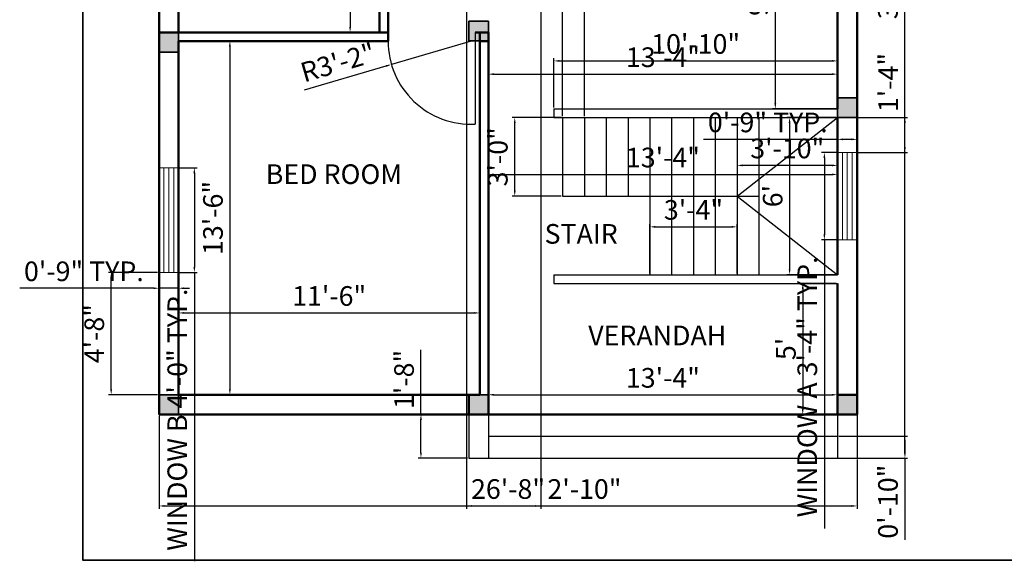
# Model space of a CAD drawing. Units: inches. Extents: x 2289 to 3796, y 1741 to 2286.
# Tile 1 of 4: x 2289 to 2741, y 1741 to 1989. Entities that reach past the tile are written whole.
import ezdxf

# ---------------------------------------------------------------- set-up
doc = ezdxf.new("R2010")
doc.units = ezdxf.units.IN
for name, color, linetype, lineweight in [('A-ANNO-DIMS', 2, 'Continuous', 18), ('A-ANNO-TTLB', 7, 'Continuous', 35), ('A-AREA-IDEN', 7, 'Continuous', 25), ('A-DOOR', 3, 'Continuous', 25), ('A-FLOR-STRS', 7, 'Continuous', 25), ('A-GLAZ', 4, 'Continuous', 18), ('A-WALL', 7, 'Continuous', 50), ('S-COLS', 1, 'Continuous', 35)]:
    doc.layers.add(name, color=color, linetype=linetype, lineweight=lineweight)
doc.styles.get("Standard").update_dxf_attribs({"font": 'arial.ttf'})
doc.dimstyles.new('ISO-25', dxfattribs={"dimtxt": 9, "dimasz": 2.5, "dimexe": 1.25, "dimexo": 0.625, "dimgap": 2, "dimtad": 1, "dimdec": 1, "dimlunit": 4, "dimtxsty": 'Standard', "dimcen": 2.5, "dimadec": 0, "dimazin": 0, "dimtfac": 1, "dimtdec": 1, "dimtmove": 0, "dimatfit": 3, "dimfxl": 1, "dimarcsym": 0})

# ---------------------------------------------------------------- blocks, each defined once
blk = doc.blocks.new('*D7')
at = {"layer": 'A-ANNO-DIMS', "color": 0, "lineweight": -2, "transparency": 16777216}
for p, q in [((2362.08, 1818.01), (2362.08, 1856.13)), ((2500.08, 1818.01), (2500.08, 1856.13)), ((2364.58, 1854.88), (2497.58, 1854.88))]:
    blk.add_line(p, q, dxfattribs=at)
at = {"layer": 'A-ANNO-DIMS', "color": 0, "transparency": 16777216}
for points in [[(2364.58, 1855.3), (2364.58, 1854.46), (2362.08, 1854.88)], [(2497.58, 1855.3), (2497.58, 1854.46), (2500.08, 1854.88)]]:
    blk.add_solid(points, dxfattribs=at)
at = {"layer": 'Defpoints', "color": 0, "transparency": 16777216}
for p in [(2500.08, 1854.88), (2362.08, 1817.39), (2500.08, 1817.39)]:
    blk.add_point(p, dxfattribs=at)
at = {"layer": 'A-ANNO-DIMS', "color": 0, "transparency": 16777216, "insert": (2431.08, 1861.48), "char_height": 9, "attachment_point": 5}
blk.add_mtext('11\'-6"', dxfattribs=at)
blk = doc.blocks.new('*D8')
at = {"layer": 'A-ANNO-DIMS', "color": 0, "lineweight": -2, "transparency": 16777216}
for p, q in [((2362.7, 1979.39), (2386.82, 1979.39)), ((2385.57, 1976.89), (2385.57, 1819.89)), ((2362.7, 1817.39), (2386.82, 1817.39))]:
    blk.add_line(p, q, dxfattribs=at)
at = {"layer": 'A-ANNO-DIMS', "color": 0, "transparency": 16777216}
for points in [[(2385.16, 1976.89), (2385.99, 1976.89), (2385.57, 1979.39)], [(2385.16, 1819.89), (2385.99, 1819.89), (2385.57, 1817.39)]]:
    blk.add_solid(points, dxfattribs=at)
at = {"layer": 'Defpoints', "color": 0, "transparency": 16777216}
for p in [(2362.08, 1979.39), (2362.08, 1817.39), (2385.57, 1817.39)]:
    blk.add_point(p, dxfattribs=at)
at = {"layer": 'A-ANNO-DIMS', "color": 0, "transparency": 16777216, "insert": (2378.98, 1898.39), "char_height": 9, "attachment_point": 5, "rotation": 90}
blk.add_mtext('13\'-6"', dxfattribs=at)
blk = doc.blocks.new('*D9')
at = {"layer": 'A-ANNO-DIMS', "color": 0, "lineweight": -2, "transparency": 16777216}
for p, q in [((2504.08, 1867.76), (2504.08, 1816.14)), ((2664.08, 1867.76), (2664.08, 1816.14)), ((2506.58, 1817.39), (2661.58, 1817.39))]:
    blk.add_line(p, q, dxfattribs=at)
at = {"layer": 'A-ANNO-DIMS', "color": 0, "transparency": 16777216}
for points in [[(2506.58, 1817.8), (2506.58, 1816.97), (2504.08, 1817.39)], [(2661.58, 1817.8), (2661.58, 1816.97), (2664.08, 1817.39)]]:
    blk.add_solid(points, dxfattribs=at)
at = {"layer": 'Defpoints', "color": 0, "transparency": 16777216}
for p in [(2504.08, 1868.39), (2664.08, 1868.39), (2664.08, 1817.39)]:
    blk.add_point(p, dxfattribs=at)
at = {"layer": 'A-ANNO-DIMS', "color": 0, "transparency": 16777216, "insert": (2584.08, 1823.98), "char_height": 9, "attachment_point": 5}
blk.add_mtext('13\'-4"', dxfattribs=at)
blk = doc.blocks.new('*D10')
at = {"layer": 'A-ANNO-DIMS', "color": 0, "lineweight": -2, "transparency": 16777216}
for p, q in [((2663.45, 1868.39), (2646.93, 1868.39)), ((2648.18, 1865.89), (2648.18, 1810.89)), ((2663.45, 1808.39), (2646.93, 1808.39))]:
    blk.add_line(p, q, dxfattribs=at)
at = {"layer": 'A-ANNO-DIMS', "color": 0, "transparency": 16777216}
for points in [[(2647.76, 1865.89), (2648.6, 1865.89), (2648.18, 1868.39)], [(2647.76, 1810.89), (2648.6, 1810.89), (2648.18, 1808.39)]]:
    blk.add_solid(points, dxfattribs=at)
at = {"layer": 'Defpoints', "color": 0, "transparency": 16777216}
for p in [(2664.08, 1868.39), (2648.18, 1808.39), (2664.08, 1808.39)]:
    blk.add_point(p, dxfattribs=at)
at = {"layer": 'A-ANNO-DIMS', "color": 0, "transparency": 16777216, "insert": (2641.6, 1838.39), "char_height": 9, "attachment_point": 5, "rotation": 90}
blk.add_mtext("5'", dxfattribs=at)
blk = doc.blocks.new('*D11')
at = {"layer": 'A-ANNO-DIMS', "color": 0, "lineweight": -2, "transparency": 16777216}
for p, q in [((2504.08, 1873.01), (2504.08, 1919.55)), ((2506.58, 1918.3), (2661.58, 1918.3)), ((2664.08, 1873.01), (2664.08, 1919.55))]:
    blk.add_line(p, q, dxfattribs=at)
at = {"layer": 'A-ANNO-DIMS', "color": 0, "transparency": 16777216}
for points in [[(2506.58, 1918.72), (2506.58, 1917.89), (2504.08, 1918.3)], [(2661.58, 1918.72), (2661.58, 1917.89), (2664.08, 1918.3)]]:
    blk.add_solid(points, dxfattribs=at)
at = {"layer": 'Defpoints', "color": 0, "transparency": 16777216}
for p in [(2664.08, 1918.3), (2504.08, 1872.39), (2664.08, 1872.39)]:
    blk.add_point(p, dxfattribs=at)
at = {"layer": 'A-ANNO-DIMS', "color": 0, "transparency": 16777216, "insert": (2584.08, 1924.9), "char_height": 9, "attachment_point": 5}
blk.add_mtext('13\'-4"', dxfattribs=at)
blk = doc.blocks.new('*D12')
at = {"layer": 'A-ANNO-DIMS', "color": 0, "lineweight": -2, "transparency": 16777216}
for p, q in [((2663.45, 1944.39), (2640.9, 1944.39)), ((2642.15, 1941.89), (2642.15, 1874.89)), ((2663.45, 1872.39), (2640.9, 1872.39))]:
    blk.add_line(p, q, dxfattribs=at)
at = {"layer": 'A-ANNO-DIMS', "color": 0, "transparency": 16777216}
for points in [[(2641.73, 1941.89), (2642.56, 1941.89), (2642.15, 1944.39)], [(2641.73, 1874.89), (2642.56, 1874.89), (2642.15, 1872.39)]]:
    blk.add_solid(points, dxfattribs=at)
at = {"layer": 'Defpoints', "color": 0, "transparency": 16777216}
for p in [(2664.08, 1944.39), (2642.15, 1872.39), (2664.08, 1872.39)]:
    blk.add_point(p, dxfattribs=at)
at = {"layer": 'A-ANNO-DIMS', "color": 0, "transparency": 16777216, "insert": (2635.55, 1908.39), "char_height": 9, "attachment_point": 5, "rotation": 90}
blk.add_mtext("6'", dxfattribs=at)
blk = doc.blocks.new('*D13')
at = {"layer": 'A-ANNO-DIMS', "color": 0, "lineweight": -2, "transparency": 16777216}
for p, q in [((2664.08, 2007.26), (2664.08, 1963)), ((2504.08, 1978.76), (2504.08, 1963)), ((2506.58, 1964.25), (2661.58, 1964.25))]:
    blk.add_line(p, q, dxfattribs=at)
at = {"layer": 'A-ANNO-DIMS', "color": 0, "transparency": 16777216}
for points in [[(2506.58, 1964.67), (2506.58, 1963.83), (2504.08, 1964.25)], [(2661.58, 1964.67), (2661.58, 1963.83), (2664.08, 1964.25)]]:
    blk.add_solid(points, dxfattribs=at)
at = {"layer": 'Defpoints', "color": 0, "transparency": 16777216}
for p in [(2664.08, 2007.89), (2504.08, 1979.39), (2664.08, 1964.25)]:
    blk.add_point(p, dxfattribs=at)
at = {"layer": 'A-ANNO-DIMS', "color": 0, "transparency": 16777216, "insert": (2584.08, 1970.85), "char_height": 9, "attachment_point": 5}
blk.add_mtext('13\'-4"', dxfattribs=at)
blk = doc.blocks.new('*D14')
at = {"layer": 'A-ANNO-DIMS', "color": 0, "lineweight": -2, "transparency": 16777216}
for p, q in [((2362.7, 2067.39), (2441.94, 2067.39)), ((2440.69, 2064.89), (2440.69, 1985.89)), ((2362.7, 1983.39), (2441.94, 1983.39))]:
    blk.add_line(p, q, dxfattribs=at)
at = {"layer": 'A-ANNO-DIMS', "color": 0, "transparency": 16777216}
for points in [[(2440.27, 2064.89), (2441.1, 2064.89), (2440.69, 2067.39)], [(2440.27, 1985.89), (2441.1, 1985.89), (2440.69, 1983.39)]]:
    blk.add_solid(points, dxfattribs=at)
at = {"layer": 'Defpoints', "color": 0, "transparency": 16777216}
for p in [(2362.08, 2067.39), (2362.08, 1983.39), (2440.69, 1983.39)]:
    blk.add_point(p, dxfattribs=at)
at = {"layer": 'A-ANNO-DIMS', "color": 0, "transparency": 16777216, "insert": (2434.19, 2025.39), "char_height": 9, "attachment_point": 5, "rotation": 90}
blk.add_mtext("7'", dxfattribs=at)
blk = doc.blocks.new('*D15')
at = {"layer": 'A-ANNO-DIMS', "color": 0, "lineweight": -2, "transparency": 16777216}
for p, q in [((2663.45, 2067.39), (2634.35, 2067.39)), ((2635.6, 2064.89), (2635.6, 1950.89)), ((2663.45, 1948.39), (2634.35, 1948.39))]:
    blk.add_line(p, q, dxfattribs=at)
at = {"layer": 'A-ANNO-DIMS', "color": 0, "transparency": 16777216}
for points in [[(2635.18, 2064.89), (2636.02, 2064.89), (2635.6, 2067.39)], [(2635.18, 1950.89), (2636.02, 1950.89), (2635.6, 1948.39)]]:
    blk.add_solid(points, dxfattribs=at)
at = {"layer": 'Defpoints', "color": 0, "transparency": 16777216}
for p in [(2664.08, 2067.39), (2635.6, 1948.39), (2664.08, 1948.39)]:
    blk.add_point(p, dxfattribs=at)
at = {"layer": 'A-ANNO-DIMS', "color": 0, "transparency": 16777216, "insert": (2629, 2007.89), "char_height": 9, "attachment_point": 5, "rotation": 90}
blk.add_mtext('9\'-11"', dxfattribs=at)
blk = doc.blocks.new('WIN-40IN')
for p, q in [((0, 40), (9, 40)), ((2.25, 40), (2.25, 0)), ((4.5, 40), (4.5, 0)), ((6.75, 40), (6.75, 0)), ((0, 0), (9, 0))]:
    blk.add_line(p, q)
blk = doc.blocks.new('WIN-48IN')
for p, q in [((0, 48), (9, 48)), ((2.25, 48), (2.25, 0)), ((4.5, 48), (4.5, 0)), ((6.75, 48), (6.75, 0)), ((0, 0), (9, 0))]:
    blk.add_line(p, q)
blk = doc.blocks.new('COL-9X9')
h = blk.add_hatch(color=256)
h.dxf.hatch_style = 1
h.paths.add_polyline_path([(0, 9), (0, 0), (9, 0), (9, 9)])
blk.add_lwpolyline([(0, 9), (9, 9), (9, 0), (0, 0)], close=True)
blk = doc.blocks.new('COL-9X9-STAIR')
h = blk.add_hatch(color=256)
h.dxf.hatch_style = 1
h.paths.add_polyline_path([(9, 0), (9, 9), (0, 9), (0, 0)])
blk.add_lwpolyline([(0.01, 9.14), (9.01, 9.14), (9.01, 0.14), (0.01, 0.14)], close=True)
blk = doc.blocks.new('*D31')
at = {"layer": 'A-ANNO-DIMS', "color": 0, "lineweight": -2, "transparency": 16777216}
for p, q in [((2663.45, 1928.39), (2656.83, 1928.39)), ((2658.08, 1925.89), (2658.08, 1890.89)), ((2663.45, 1888.39), (2656.83, 1888.39)), ((2658.08, 1888.39), (2658.08, 1756.12))]:
    blk.add_line(p, q, dxfattribs=at)
at = {"layer": 'A-ANNO-DIMS', "color": 0, "transparency": 16777216}
for points in [[(2657.66, 1925.89), (2658.49, 1925.89), (2658.08, 1928.39)], [(2657.66, 1890.89), (2658.49, 1890.89), (2658.08, 1888.39)]]:
    blk.add_solid(points, dxfattribs=at)
at = {"layer": 'Defpoints', "color": 0, "transparency": 16777216}
for p in [(2664.08, 1928.39), (2658.08, 1888.39), (2664.08, 1888.39)]:
    blk.add_point(p, dxfattribs=at)
at = {"layer": 'A-ANNO-DIMS', "color": 0, "transparency": 16777216, "insert": (2651.42, 1821), "char_height": 9, "attachment_point": 5, "rotation": 90}
blk.add_mtext('WINDOW A 3\'-4" TYP.', dxfattribs=at)
blk = doc.blocks.new('*D32')
at = {"layer": 'A-ANNO-DIMS', "color": 0, "lineweight": -2, "transparency": 16777216}
for p, q in [((2664.08, 1934.39), (2602.72, 1934.39)), ((2664.08, 1929.01), (2664.08, 1935.64)), ((2670.58, 1934.39), (2666.58, 1934.39)), ((2673.08, 1929.01), (2673.08, 1935.64))]:
    blk.add_line(p, q, dxfattribs=at)
at = {"layer": 'A-ANNO-DIMS', "color": 0, "transparency": 16777216}
for points in [[(2666.58, 1934.8), (2666.58, 1933.97), (2664.08, 1934.39)], [(2670.58, 1934.8), (2670.58, 1933.97), (2673.08, 1934.39)]]:
    blk.add_solid(points, dxfattribs=at)
at = {"layer": 'Defpoints', "color": 0, "transparency": 16777216}
for p in [(2664.08, 1934.39), (2664.08, 1928.39), (2673.08, 1928.39)]:
    blk.add_point(p, dxfattribs=at)
at = {"layer": 'A-ANNO-DIMS', "color": 0, "transparency": 16777216, "insert": (2632.15, 1940.98), "char_height": 9, "attachment_point": 5}
blk.add_mtext('0\'-9" TYP.', dxfattribs=at)
blk = doc.blocks.new('*D33')
at = {"layer": 'A-ANNO-DIMS', "color": 0, "lineweight": -2, "transparency": 16777216}
for p, q in [((2362.7, 1921.39), (2370.53, 1921.39)), ((2369.28, 1918.89), (2369.28, 1875.89)), ((2362.7, 1873.39), (2370.53, 1873.39)), ((2369.28, 1873.39), (2369.28, 1741.12))]:
    blk.add_line(p, q, dxfattribs=at)
at = {"layer": 'A-ANNO-DIMS', "color": 0, "transparency": 16777216}
for points in [[(2368.86, 1918.89), (2369.69, 1918.89), (2369.28, 1921.39)], [(2368.86, 1875.89), (2369.69, 1875.89), (2369.28, 1873.39)]]:
    blk.add_solid(points, dxfattribs=at)
at = {"layer": 'Defpoints', "color": 0, "transparency": 16777216}
for p in [(2362.08, 1921.39), (2362.08, 1873.39), (2369.28, 1873.39)]:
    blk.add_point(p, dxfattribs=at)
at = {"layer": 'A-ANNO-DIMS', "color": 0, "transparency": 16777216, "insert": (2362.62, 1806), "char_height": 9, "attachment_point": 5, "rotation": 90}
blk.add_mtext('WINDOW B 4\'-0" TYP.', dxfattribs=at)
blk = doc.blocks.new('*D34')
at = {"layer": 'A-ANNO-DIMS', "color": 0, "lineweight": -2, "transparency": 16777216}
for p, q in [((2353.08, 1872.76), (2353.08, 1864.94)), ((2362.08, 1872.76), (2362.08, 1864.94)), ((2350.58, 1866.19), (2289.22, 1866.19)), ((2362.08, 1866.19), (2353.08, 1866.19)), ((2364.58, 1866.19), (2367.08, 1866.19))]:
    blk.add_line(p, q, dxfattribs=at)
at = {"layer": 'A-ANNO-DIMS', "color": 0, "transparency": 16777216}
for points in [[(2350.58, 1866.6), (2350.58, 1865.77), (2353.08, 1866.19)], [(2364.58, 1866.6), (2364.58, 1865.77), (2362.08, 1866.19)]]:
    blk.add_solid(points, dxfattribs=at)
at = {"layer": 'Defpoints', "color": 0, "transparency": 16777216}
for p in [(2353.08, 1873.39), (2362.08, 1873.39), (2353.08, 1866.19)]:
    blk.add_point(p, dxfattribs=at)
at = {"layer": 'A-ANNO-DIMS', "color": 0, "transparency": 16777216, "insert": (2318.65, 1872.78), "char_height": 9, "attachment_point": 5}
blk.add_mtext('0\'-9" TYP.', dxfattribs=at)
blk = doc.blocks.new('*D35')
at = {"layer": 'A-ANNO-DIMS', "color": 0, "lineweight": -2, "transparency": 16777216}
for p, q in [((2353.08, 1807.76), (2353.08, 1765.21)), ((2673.08, 1787.76), (2673.08, 1765.21)), ((2355.58, 1766.46), (2670.58, 1766.46))]:
    blk.add_line(p, q, dxfattribs=at)
at = {"layer": 'A-ANNO-DIMS', "color": 0, "transparency": 16777216}
for points in [[(2355.58, 1766.88), (2355.58, 1766.04), (2353.08, 1766.46)], [(2670.58, 1766.88), (2670.58, 1766.04), (2673.08, 1766.46)]]:
    blk.add_solid(points, dxfattribs=at)
at = {"layer": 'Defpoints', "color": 0, "transparency": 16777216}
for p in [(2353.08, 1808.39), (2673.08, 1788.39), (2673.08, 1766.46)]:
    blk.add_point(p, dxfattribs=at)
at = {"layer": 'A-ANNO-DIMS', "color": 0, "transparency": 16777216, "insert": (2513.08, 1773.06), "char_height": 9, "attachment_point": 5}
blk.add_mtext('26\'-8"', dxfattribs=at)
blk = doc.blocks.new('*D36')
at = {"layer": 'A-ANNO-DIMS', "color": 0, "lineweight": -2, "transparency": 16777216}
for p, q in [((2673.7, 2224.39), (2696.25, 2224.39)), ((2695, 1790.89), (2695, 2221.89)), ((2673.7, 1788.39), (2696.25, 1788.39))]:
    blk.add_line(p, q, dxfattribs=at)
at = {"layer": 'A-ANNO-DIMS', "color": 0, "transparency": 16777216}
for points in [[(2694.59, 2221.89), (2695.42, 2221.89), (2695, 2224.39)], [(2694.59, 1790.89), (2695.42, 1790.89), (2695, 1788.39)]]:
    blk.add_solid(points, dxfattribs=at)
at = {"layer": 'Defpoints', "color": 0, "transparency": 16777216}
for p in [(2673.08, 2224.39), (2695, 2224.39), (2673.08, 1788.39)]:
    blk.add_point(p, dxfattribs=at)
at = {"layer": 'A-ANNO-DIMS', "color": 0, "transparency": 16777216, "insert": (2688.4, 2006.39), "char_height": 9, "attachment_point": 5, "rotation": 90}
blk.add_mtext('36\'-4"', dxfattribs=at)
blk = doc.blocks.new('*D37')
at = {"layer": 'A-ANNO-DIMS', "color": 0, "lineweight": -2, "transparency": 16777216}
for p, q in [((2473.15, 1808.39), (2473.15, 1837.96)), ((2494.45, 1808.39), (2471.9, 1808.39)), ((2473.15, 1790.89), (2473.15, 1805.89)), ((2494.45, 1788.39), (2471.9, 1788.39))]:
    blk.add_line(p, q, dxfattribs=at)
at = {"layer": 'A-ANNO-DIMS', "color": 0, "transparency": 16777216}
for points in [[(2472.74, 1805.89), (2473.57, 1805.89), (2473.15, 1808.39)], [(2472.74, 1790.89), (2473.57, 1790.89), (2473.15, 1788.39)]]:
    blk.add_solid(points, dxfattribs=at)
at = {"layer": 'Defpoints', "color": 0, "transparency": 16777216}
for p in [(2473.15, 1808.39), (2495.08, 1808.39), (2495.08, 1788.39)]:
    blk.add_point(p, dxfattribs=at)
at = {"layer": 'A-ANNO-DIMS', "color": 0, "transparency": 16777216, "insert": (2466.56, 1824.42), "char_height": 9, "attachment_point": 5, "rotation": 90}
blk.add_mtext('1\'-8"', dxfattribs=at)
blk = doc.blocks.new('*D40')
at = {"layer": 'A-ANNO-DIMS', "color": 0, "lineweight": -2, "transparency": 16777216}
for p, q in [((2352.45, 1873.39), (2329.9, 1873.39)), ((2331.15, 1819.89), (2331.15, 1870.89)), ((2352.45, 1817.39), (2329.9, 1817.39))]:
    blk.add_line(p, q, dxfattribs=at)
at = {"layer": 'A-ANNO-DIMS', "color": 0, "transparency": 16777216}
for points in [[(2330.74, 1870.89), (2331.57, 1870.89), (2331.15, 1873.39)], [(2330.74, 1819.89), (2331.57, 1819.89), (2331.15, 1817.39)]]:
    blk.add_solid(points, dxfattribs=at)
at = {"layer": 'Defpoints', "color": 0, "transparency": 16777216}
for p in [(2331.15, 1873.39), (2353.08, 1873.39), (2353.08, 1817.39)]:
    blk.add_point(p, dxfattribs=at)
at = {"layer": 'A-ANNO-DIMS', "color": 0, "transparency": 16777216, "insert": (2324.56, 1845.39), "char_height": 9, "attachment_point": 5, "rotation": 90}
blk.add_mtext('4\'-8"', dxfattribs=at)
blk = doc.blocks.new('*D43')
at = {"layer": 'A-ANNO-DIMS', "color": 0, "lineweight": -2, "transparency": 16777216}
for p, q in [((2695, 1944.39), (2695, 1973.96)), ((2673.7, 1944.39), (2696.25, 1944.39)), ((2695, 1930.89), (2695, 1941.89)), ((2673.7, 1928.39), (2696.25, 1928.39))]:
    blk.add_line(p, q, dxfattribs=at)
at = {"layer": 'A-ANNO-DIMS', "color": 0, "transparency": 16777216}
for points in [[(2694.59, 1941.89), (2695.42, 1941.89), (2695, 1944.39)], [(2694.59, 1930.89), (2695.42, 1930.89), (2695, 1928.39)]]:
    blk.add_solid(points, dxfattribs=at)
at = {"layer": 'Defpoints', "color": 0, "transparency": 16777216}
for p in [(2673.08, 1944.39), (2695, 1944.39), (2673.08, 1928.39)]:
    blk.add_point(p, dxfattribs=at)
at = {"layer": 'A-ANNO-DIMS', "color": 0, "transparency": 16777216, "insert": (2688.48, 1960.42), "char_height": 9, "attachment_point": 5, "rotation": 90}
blk.add_mtext('1\'-4"', dxfattribs=at)
blk = doc.blocks.new('*D46')
at = {"layer": 'A-ANNO-DIMS', "color": 0, "lineweight": -2, "transparency": 16777216}
for p, q in [((2494.08, 2126.76), (2494.08, 1765.21)), ((2528.08, 2126.76), (2528.08, 1765.21)), ((2496.58, 1766.46), (2525.58, 1766.46)), ((2528.08, 1766.46), (2565.65, 1766.46))]:
    blk.add_line(p, q, dxfattribs=at)
at = {"layer": 'A-ANNO-DIMS', "color": 0, "transparency": 16777216}
for points in [[(2496.58, 1766.88), (2496.58, 1766.04), (2494.08, 1766.46)], [(2525.58, 1766.88), (2525.58, 1766.04), (2528.08, 1766.46)]]:
    blk.add_solid(points, dxfattribs=at)
at = {"layer": 'Defpoints', "color": 0, "transparency": 16777216}
for p in [(2494.08, 2127.39), (2528.08, 2127.39), (2528.08, 1766.46)]:
    blk.add_point(p, dxfattribs=at)
at = {"layer": 'A-ANNO-DIMS', "color": 0, "transparency": 16777216, "insert": (2548.11, 1773.06), "char_height": 9, "attachment_point": 5}
blk.add_mtext('2\'-10"', dxfattribs=at)
blk = doc.blocks.new('*D48')
at = {"layer": 'A-ANNO-DIMS', "color": 0, "lineweight": -2, "transparency": 16777216}
for p, q in [((2538.08, 1945.01), (2538.08, 2247.56)), ((2540.58, 2246.31), (2545.58, 2246.31)), ((2548.08, 1945.01), (2548.08, 2247.56)), ((2548.08, 2246.31), (2585.49, 2246.31))]:
    blk.add_line(p, q, dxfattribs=at)
at = {"layer": 'A-ANNO-DIMS', "color": 0, "transparency": 16777216}
for points in [[(2540.58, 2246.73), (2540.58, 2245.89), (2538.08, 2246.31)], [(2545.58, 2246.73), (2545.58, 2245.89), (2548.08, 2246.31)]]:
    blk.add_solid(points, dxfattribs=at)
at = {"layer": 'Defpoints', "color": 0, "transparency": 16777216}
for p in [(2548.08, 2246.31), (2538.08, 1944.39), (2548.08, 1944.39)]:
    blk.add_point(p, dxfattribs=at)
at = {"layer": 'A-ANNO-DIMS', "color": 0, "transparency": 16777216, "insert": (2568.04, 2252.91), "char_height": 9, "attachment_point": 5}
blk.add_mtext('0\'-10"', dxfattribs=at)
blk = doc.blocks.new('*D49')
at = {"layer": 'A-ANNO-DIMS', "color": 0, "lineweight": -2, "transparency": 16777216}
for p, q in [((2537.45, 1944.39), (2514.9, 1944.39)), ((2516.15, 1910.89), (2516.15, 1941.89)), ((2537.45, 1908.39), (2514.9, 1908.39))]:
    blk.add_line(p, q, dxfattribs=at)
at = {"layer": 'A-ANNO-DIMS', "color": 0, "transparency": 16777216}
for points in [[(2515.74, 1941.89), (2516.57, 1941.89), (2516.15, 1944.39)], [(2515.74, 1910.89), (2516.57, 1910.89), (2516.15, 1908.39)]]:
    blk.add_solid(points, dxfattribs=at)
at = {"layer": 'Defpoints', "color": 0, "transparency": 16777216}
for p in [(2516.15, 1944.39), (2538.08, 1944.39), (2538.08, 1908.39)]:
    blk.add_point(p, dxfattribs=at)
at = {"layer": 'A-ANNO-DIMS', "color": 0, "transparency": 16777216, "insert": (2509.55, 1926.39), "char_height": 9, "attachment_point": 5, "rotation": 90}
blk.add_mtext('3\'-0"', dxfattribs=at)
blk = doc.blocks.new('*D50')
at = {"layer": 'A-ANNO-DIMS', "color": 0, "lineweight": -2, "transparency": 16777216}
for p, q in [((2618.08, 1943.76), (2618.08, 1921.21)), ((2664.08, 1943.76), (2664.08, 1921.21)), ((2661.58, 1922.46), (2620.58, 1922.46))]:
    blk.add_line(p, q, dxfattribs=at)
at = {"layer": 'A-ANNO-DIMS', "color": 0, "transparency": 16777216}
for points in [[(2620.58, 1922.88), (2620.58, 1922.04), (2618.08, 1922.46)], [(2661.58, 1922.88), (2661.58, 1922.04), (2664.08, 1922.46)]]:
    blk.add_solid(points, dxfattribs=at)
at = {"layer": 'Defpoints', "color": 0, "transparency": 16777216}
for p in [(2618.08, 1944.39), (2664.08, 1944.39), (2618.08, 1922.46)]:
    blk.add_point(p, dxfattribs=at)
at = {"layer": 'A-ANNO-DIMS', "color": 0, "transparency": 16777216, "insert": (2641.08, 1929.06), "char_height": 9, "attachment_point": 5}
blk.add_mtext('3\'-10"', dxfattribs=at)
blk = doc.blocks.new('*D51')
at = {"layer": 'A-ANNO-DIMS', "color": 0, "lineweight": -2, "transparency": 16777216}
for p, q in [((2578.08, 1873.01), (2578.08, 1895.56)), ((2580.58, 1894.31), (2615.58, 1894.31)), ((2618.08, 1873.01), (2618.08, 1895.56))]:
    blk.add_line(p, q, dxfattribs=at)
at = {"layer": 'A-ANNO-DIMS', "color": 0, "transparency": 16777216}
for points in [[(2580.58, 1894.73), (2580.58, 1893.89), (2578.08, 1894.31)], [(2615.58, 1894.73), (2615.58, 1893.89), (2618.08, 1894.31)]]:
    blk.add_solid(points, dxfattribs=at)
at = {"layer": 'Defpoints', "color": 0, "transparency": 16777216}
for p in [(2618.08, 1894.31), (2578.08, 1872.39), (2618.08, 1872.39)]:
    blk.add_point(p, dxfattribs=at)
at = {"layer": 'A-ANNO-DIMS', "color": 0, "transparency": 16777216, "insert": (2598.08, 1900.91), "char_height": 9, "attachment_point": 5}
blk.add_mtext('3\'-4"', dxfattribs=at)
blk = doc.blocks.new('*D52')
at = {"layer": 'A-ANNO-DIMS', "color": 0, "lineweight": -2, "transparency": 16777216}
for p, q in [((2534.08, 1949.01), (2534.08, 1971.56)), ((2536.58, 1970.31), (2661.58, 1970.31)), ((2664.08, 1949.01), (2664.08, 1971.56))]:
    blk.add_line(p, q, dxfattribs=at)
at = {"layer": 'A-ANNO-DIMS', "color": 0, "transparency": 16777216}
for points in [[(2536.58, 1970.73), (2536.58, 1969.89), (2534.08, 1970.31)], [(2661.58, 1970.73), (2661.58, 1969.89), (2664.08, 1970.31)]]:
    blk.add_solid(points, dxfattribs=at)
at = {"layer": 'Defpoints', "color": 0, "transparency": 16777216}
for p in [(2664.08, 1970.31), (2534.08, 1948.39), (2664.08, 1948.39)]:
    blk.add_point(p, dxfattribs=at)
at = {"layer": 'A-ANNO-DIMS', "color": 0, "transparency": 16777216, "insert": (2599.08, 1976.91), "char_height": 9, "attachment_point": 5}
blk.add_mtext('10\'-10"', dxfattribs=at)
blk = doc.blocks.new('*D53')
at = {"layer": 'A-ANNO-DIMS', "color": 0, "lineweight": -2, "transparency": 16777216}
for p, q in [((2664.7, 1798.39), (2696.25, 1798.39)), ((2695, 1795.89), (2695, 1790.89)), ((2664.7, 1788.39), (2696.25, 1788.39)), ((2695, 1788.39), (2695, 1750.97))]:
    blk.add_line(p, q, dxfattribs=at)
at = {"layer": 'A-ANNO-DIMS', "color": 0, "transparency": 16777216}
for points in [[(2694.59, 1795.89), (2695.42, 1795.89), (2695, 1798.39)], [(2694.59, 1790.89), (2695.42, 1790.89), (2695, 1788.39)]]:
    blk.add_solid(points, dxfattribs=at)
at = {"layer": 'Defpoints', "color": 0, "transparency": 16777216}
for p in [(2664.08, 1798.39), (2664.08, 1788.39), (2695, 1788.39)]:
    blk.add_point(p, dxfattribs=at)
at = {"layer": 'A-ANNO-DIMS', "color": 0, "transparency": 16777216, "insert": (2688.41, 1768.43), "char_height": 9, "attachment_point": 5, "rotation": 90}
blk.add_mtext('0\'-10"', dxfattribs=at)
blk = doc.blocks.new('*D78')
at = {"layer": 'A-ANNO-DIMS', "color": 0, "lineweight": -2, "transparency": 16777216}
for p, q in [((2496.13, 1979.39), (2459.61, 1968.7)), ((2419.74, 1957.04), (2457.21, 1968))]:
    blk.add_line(p, q, dxfattribs=at)
at = {"layer": 'A-ANNO-DIMS', "color": 0, "transparency": 16777216}
blk.add_solid([(2457.09, 1968.4), (2457.33, 1967.6), (2459.61, 1968.7)], dxfattribs=at)
at = {"layer": 'Defpoints', "color": 0, "transparency": 16777216}
for p in [(2496.13, 1979.39), (2459.61, 1968.7)]:
    blk.add_point(p, dxfattribs=at)
at = {"layer": 'A-ANNO-DIMS', "color": 0, "transparency": 16777216, "insert": (2435.42, 1968.5), "char_height": 9, "attachment_point": 5, "rotation": 16.3066}
blk.add_mtext('R3\'-2"', dxfattribs=at)

msp = doc.modelspace()

# ---------------------------------------------------------------- linework, layer by layer
at = {"layer": 'A-ANNO-TTLB'}
msp.add_lwpolyline([(2318.16, 2245.19), (3750.19, 2245.19), (3750.19, 1741.69), (2318.16, 1741.69)], close=True, dxfattribs=at)
at = {"layer": 'A-DOOR'}
msp.add_line((2498.08, 1983.39), (2498.08, 1941.39), dxfattribs=at)
msp.add_arc((2496.13, 1979.39), 38.05, 180, 272.9376, dxfattribs=at)
at = {"layer": 'A-FLOR-STRS'}
for p, q in [((2534.08, 1948.39), (2534.08, 1944.39)), ((2534.08, 1948.39), (2664.08, 1948.39)), ((2534.08, 1944.39), (2673.08, 1944.39)), ((2538.08, 1944.39), (2538.08, 1908.39)), ((2548.08, 1944.39), (2548.08, 1908.39)), ((2558.08, 1944.39), (2558.08, 1908.39)), ((2568.08, 1944.39), (2568.08, 1908.39)), ((2578.08, 1944.39), (2578.08, 1872.39)), ((2588.08, 1944.39), (2588.08, 1872.39)), ((2598.08, 1944.39), (2598.08, 1872.39)), ((2608.08, 1944.39), (2608.08, 1872.39)), ((2618.08, 1944.39), (2618.08, 1872.39)), ((2618.08, 1908.39), (2664.08, 1944.39)), ((2628.08, 1944.39), (2628.08, 1872.39)), ((2538.08, 1908.39), (2628.08, 1908.39)), ((2618.08, 1908.39), (2664.08, 1872.39)), ((2534.08, 1872.39), (2664.08, 1872.39)), ((2534.08, 1872.39), (2534.08, 1868.39)), ((2534.08, 1868.39), (2664.08, 1868.39)), ((2495.08, 1808.39), (2495.08, 1788.39)), ((2504.08, 1808.39), (2504.08, 1788.39)), ((2664.08, 1808.39), (2664.08, 1788.39)), ((2673.08, 1808.39), (2673.08, 1788.39)), ((2504.08, 1798.39), (2664.08, 1798.39)), ((2495.08, 1788.39), (2673.08, 1788.39))]:
    msp.add_line(p, q, dxfattribs=at)
at = {"layer": 'A-WALL'}
for p, q in [((2353.08, 2224.39), (2353.08, 1808.39)), ((2673.08, 2224.39), (2673.08, 1808.39)), ((2362.08, 2067.39), (2362.08, 1983.39)), ((2664.08, 2067.39), (2664.08, 1948.39)), ((2454.08, 2023.39), (2454.08, 1983.39)), ((2458.08, 2023.39), (2458.08, 1979.39)), ((2353.08, 1983.39), (2458.08, 1983.39)), ((2498.08, 1983.39), (2500.08, 1983.39)), ((2500.08, 1983.39), (2500.08, 1817.39)), ((2500.08, 1983.39), (2504.08, 1983.39)), ((2504.08, 1983.39), (2504.08, 1868.39)), ((2362.08, 1979.39), (2458.08, 1979.39)), ((2362.08, 1979.39), (2362.08, 1817.39)), ((2500.08, 1979.39), (2504.08, 1979.39)), ((2664.08, 1944.39), (2664.08, 1872.39)), ((2504.08, 1868.39), (2504.08, 1808.39)), ((2664.08, 1868.39), (2664.08, 1808.39)), ((2362.08, 1817.39), (2500.08, 1817.39)), ((2495.08, 1817.39), (2495.08, 1808.39)), ((2664.08, 1817.39), (2673.08, 1817.39)), ((2353.08, 1808.39), (2673.08, 1808.39))]:
    msp.add_line(p, q, dxfattribs=at)

# ---------------------------------------------------------------- block references
at = {"layer": 'A-GLAZ', "rotation": 180}
for name, p in [('WIN-40IN', (2673.08, 1928.39)), ('WIN-48IN', (2362.08, 1921.39))]:
    msp.add_blockref(name, p, dxfattribs=at)
at = {"layer": 'S-COLS'}
for name, p in [('COL-9X9-STAIR', (2495.06, 1979.36)), ('COL-9X9', (2353.08, 1974.39)), ('COL-9X9', (2664.08, 1944.39)), ('COL-9X9', (2353.08, 1808.39)), ('COL-9X9', (2495.08, 1808.39)), ('COL-9X9', (2664.08, 1808.39))]:
    msp.add_blockref(name, p, dxfattribs=at)

# ---------------------------------------------------------------- texts
at = {"layer": 'A-AREA-IDEN'}
for s, p in [('BED ROOM', (2402.02, 1913.94)), ('        STAIR', (2507.82, 1886.6)), ('VERANDAH', (2549.84, 1840.06))]:
    msp.add_text(s, height=9, dxfattribs=at).set_placement(p)

# ---------------------------------------------------------------- dimensions: what is measured, and where the dimension line sits
at = {"layer": 'A-ANNO-DIMS'}
for base, p1, p2, override, picture, middle in [((2548.08, 2246.31), (2538.08, 1944.39), (2548.08, 1944.39), {"dimdec": 1, "dimlfac": 1, "dimrnd": 0, "dimzin": 1, "dimdsep": 46, "dimlunit": 4, "dimfrac": 2}, '*D48', (2568.04, 2252.91)), ((2528.08, 1766.46), (2494.08, 2127.39), (2528.08, 2127.39), {"dimdec": 1, "dimlfac": 1, "dimrnd": 0, "dimzin": 1, "dimdsep": 46, "dimlunit": 4, "dimfrac": 2}, '*D46', (2548.11, 1773.06)), ((2664.08, 1964.25), (2504.08, 1979.39), (2664.08, 2007.89), {"dimclrd": 0, "dimclre": 0, "dimclrt": 0}, '*D13', (2584.08, 1970.85)), ((2664.08, 1970.31), (2534.08, 1948.39), (2664.08, 1948.39), {"dimdec": 1, "dimlfac": 1, "dimrnd": 0, "dimzin": 1, "dimdsep": 46, "dimlunit": 4, "dimfrac": 2}, '*D52', (2599.08, 1976.91)), ((2664.08, 1918.3), (2504.08, 1872.39), (2664.08, 1872.39), {"dimclrd": 0, "dimclre": 0, "dimclrt": 0}, '*D11', (2584.08, 1924.9)), ((2618.08, 1894.31), (2578.08, 1872.39), (2618.08, 1872.39), {"dimdec": 1, "dimlfac": 1, "dimrnd": 0, "dimzin": 1, "dimdsep": 46, "dimlunit": 4, "dimfrac": 2}, '*D51', (2598.08, 1900.91)), ((2500.08, 1854.88), (2362.08, 1817.39), (2500.08, 1817.39), {"dimclrd": 0, "dimclre": 0, "dimclrt": 0}, '*D7', (2431.08, 1861.48)), ((2664.08, 1817.39), (2504.08, 1868.39), (2664.08, 1868.39), {"dimclrd": 0, "dimclre": 0, "dimclrt": 0}, '*D9', (2584.08, 1823.98)), ((2673.08, 1766.46), (2353.08, 1808.39), (2673.08, 1788.39), {"dimdec": 1, "dimlfac": 1, "dimrnd": 0, "dimzin": 1, "dimdsep": 46, "dimlunit": 4, "dimfrac": 2}, '*D35', (2513.08, 1773.06))]:
    dim = msp.add_linear_dim(base=base, p1=p1, p2=p2, dimstyle='ISO-25', override=override, dxfattribs=at)
    dim.commit()
    dim.dimension.update_dxf_attribs({"geometry": picture, "text_midpoint": middle})
for base, p1, p2, angle, override, picture, middle in [((2695, 2224.39), (2673.08, 1788.39), (2673.08, 2224.39), 90, {"dimdec": 1, "dimlfac": 1, "dimrnd": 0, "dimzin": 1, "dimdsep": 46, "dimlunit": 4, "dimfrac": 2}, '*D36', (2688.4, 2006.39)), ((2440.69, 1983.39), (2362.08, 2067.39), (2362.08, 1983.39), 90, {"dimclrd": 0, "dimclre": 0, "dimclrt": 0}, '*D14', (2434.19, 2025.39)), ((2635.6, 1948.39), (2664.08, 2067.39), (2664.08, 1948.39), 90, {"dimclrd": 0, "dimclre": 0, "dimclrt": 0}, '*D15', (2629, 2007.89)), ((2385.57, 1817.39), (2362.08, 1979.39), (2362.08, 1817.39), 90, {"dimclrd": 0, "dimclre": 0, "dimclrt": 0}, '*D8', (2378.98, 1898.39)), ((2695, 1944.39), (2673.08, 1928.39), (2673.08, 1944.39), 90, {"dimdec": 1, "dimlfac": 1, "dimrnd": 0, "dimzin": 1, "dimdsep": 46, "dimlunit": 4, "dimfrac": 2}, '*D43', (2688.48, 1960.42)), ((2516.15, 1944.39), (2538.08, 1908.39), (2538.08, 1944.39), 90, {"dimdec": 1, "dimlfac": 1, "dimrnd": 0, "dimzin": 1, "dimdsep": 46, "dimlunit": 4, "dimfrac": 2}, '*D49', (2509.55, 1926.39)), ((2618.08, 1922.46), (2664.08, 1944.39), (2618.08, 1944.39), 180, {"dimdec": 1, "dimlfac": 1, "dimrnd": 0, "dimzin": 1, "dimdsep": 46, "dimlunit": 4, "dimfrac": 2}, '*D50', (2641.08, 1929.06)), ((2642.15, 1872.39), (2664.08, 1944.39), (2664.08, 1872.39), 90, {"dimclrd": 0, "dimclre": 0, "dimclrt": 0}, '*D12', (2635.55, 1908.39)), ((2331.15, 1873.39), (2353.08, 1817.39), (2353.08, 1873.39), 90, {"dimdec": 1, "dimlfac": 1, "dimrnd": 0, "dimzin": 1, "dimdsep": 46, "dimlunit": 4, "dimfrac": 2}, '*D40', (2324.56, 1845.39)), ((2648.18, 1808.39), (2664.08, 1868.39), (2664.08, 1808.39), 90, {"dimclrd": 0, "dimclre": 0, "dimclrt": 0}, '*D10', (2641.6, 1838.39)), ((2473.15, 1808.39), (2495.08, 1788.39), (2495.08, 1808.39), 90, {"dimdec": 1, "dimlfac": 1, "dimrnd": 0, "dimzin": 1, "dimdsep": 46, "dimlunit": 4, "dimfrac": 2}, '*D37', (2466.56, 1824.42)), ((2695, 1788.39), (2664.08, 1798.39), (2664.08, 1788.39), 90, {"dimdec": 1, "dimlfac": 1, "dimrnd": 0, "dimzin": 1, "dimdsep": 46, "dimlunit": 4, "dimfrac": 2}, '*D53', (2688.41, 1768.43))]:
    dim = msp.add_linear_dim(base=base, p1=p1, p2=p2, angle=angle, dimstyle='ISO-25', override=override, dxfattribs=at)
    dim.commit()
    dim.dimension.update_dxf_attribs({"geometry": picture, "text_midpoint": middle})
dim = msp.add_radius_dim(center=(2496.1272, 1979.3858), mpoint=(2459.6078, 1968.7023), dimstyle='ISO-25', override={"dimdec": 1, "dimlfac": 1, "dimrnd": 0, "dimzin": 1, "dimdsep": 46, "dimlunit": 4, "dimfrac": 2}, dxfattribs=at)
dim.commit()
dim.dimension.update_dxf_attribs({"geometry": '*D78', "text_midpoint": (2435.4225, 1968.5018)})
for base, p1, p2, angle, text, picture, middle in [((2664.08, 1934.39), (2673.08, 1928.39), (2664.08, 1928.39), 180, '<> TYP.', '*D32', (2632.15, 1940.98)), ((2658.08, 1888.39), (2664.08, 1928.39), (2664.08, 1888.39), 270, 'WINDOW A <> TYP.', '*D31', (2651.42, 1821)), ((2369.28, 1873.39), (2362.08, 1921.39), (2362.08, 1873.39), 270, 'WINDOW B <> TYP.', '*D33', (2362.62, 1806)), ((2353.08, 1866.19), (2362.08, 1873.39), (2353.08, 1873.39), 180, '<> TYP.', '*D34', (2318.65, 1872.78))]:
    dim = msp.add_linear_dim(base=base, p1=p1, p2=p2, angle=angle, text=text, dimstyle='ISO-25', override={"dimdec": 1, "dimlfac": 1, "dimrnd": 0, "dimzin": 1, "dimdsep": 46, "dimlunit": 4, "dimfrac": 2}, dxfattribs=at)
    dim.commit()
    dim.dimension.update_dxf_attribs({"geometry": picture, "text_midpoint": middle})

doc.saveas('drawing.dxf')
